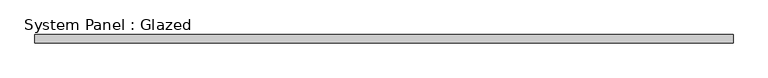
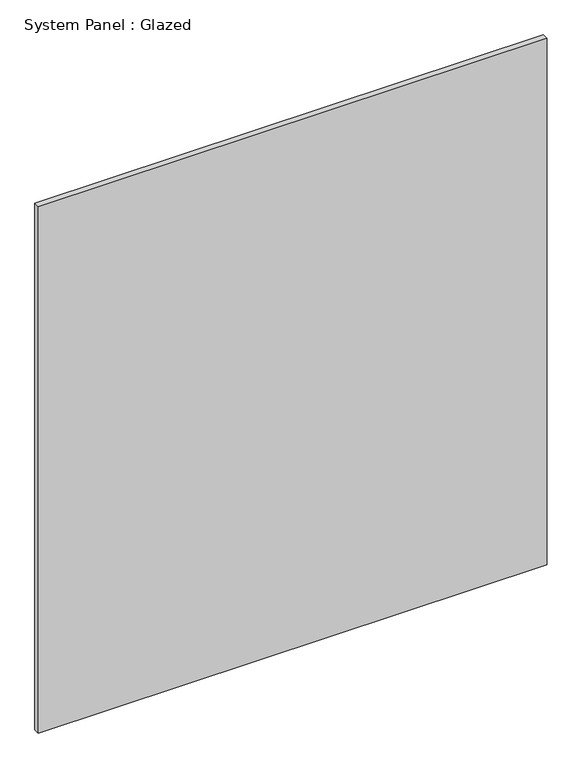
"""IFC4 building model written with IfcOpenShell, lengths in millimetres: plate geometry, System Panel : Glazed."""

from ifc_helpers import new_model, si_unit, origin, origin_with_axes, place, context, project, spatial, polyline, outline, extrude, source, transform, mapped, element, save


def system_panel_glazed_48ffcee9(model_context):
    return source(origin(), model_context, "Body", "SweptSolid", [
        extrude(outline(polyline([(1057.275, 19.05), (-1057.275, 19.05), (-1057.275, 44.45), (1057.275, 44.45), (1057.275, 19.05)])), origin_with_axes(), (0.0, 0.0, 1.0), 2311.4),
    ])


if __name__ == "__main__":
    model = new_model("IFC4")
    model_context = context("Model", 3, world=origin())
    ifc_project = project(units=[si_unit("LENGTHUNIT", "METRE", prefix="MILLI")], contexts=[model_context])
    site = spatial("IfcSite", under=ifc_project)
    building = spatial("IfcBuilding", under=site)
    placement = place(None, origin())
    system_panel_glazed_shape = system_panel_glazed_48ffcee9(model_context)
    element("IfcPlate", 1, ObjectType="System Panel : Glazed", at=placement, inside=building, context=model_context, shape_type="MappedRepresentation", body=[
        mapped(system_panel_glazed_shape, transform((0.0, 0.0, 0.0), x_axis=(1.0, 0.0, 0.0), y_axis=(0.0, 1.0, 0.0), z_axis=(0.0, 0.0, 1.0))),
    ])
    save(model, "model.ifc")

# Revit data of these elements
# Type "System Panel : Glazed"
#   Construction Type Id = "GSP4R"
#   Analytic Construction = "1/8 in Pilkington single glazing"
#   Visual Light Transmittance = 0.9
#   Solar Heat Gain Coefficient = 0.86
#   Heat Transfer Coefficient (U) = 1.18115 BTU/(h·ft²·°F)
# Element 1 (IfcPlate, "System Panel : Glazed")
#   Materials on its faces: "Glass"
# Materials
#   "Glass": class "Glass", colour RGB 0 128 192, transparency 0.75, Description = "Soda Lime Glass", Cost = 0
